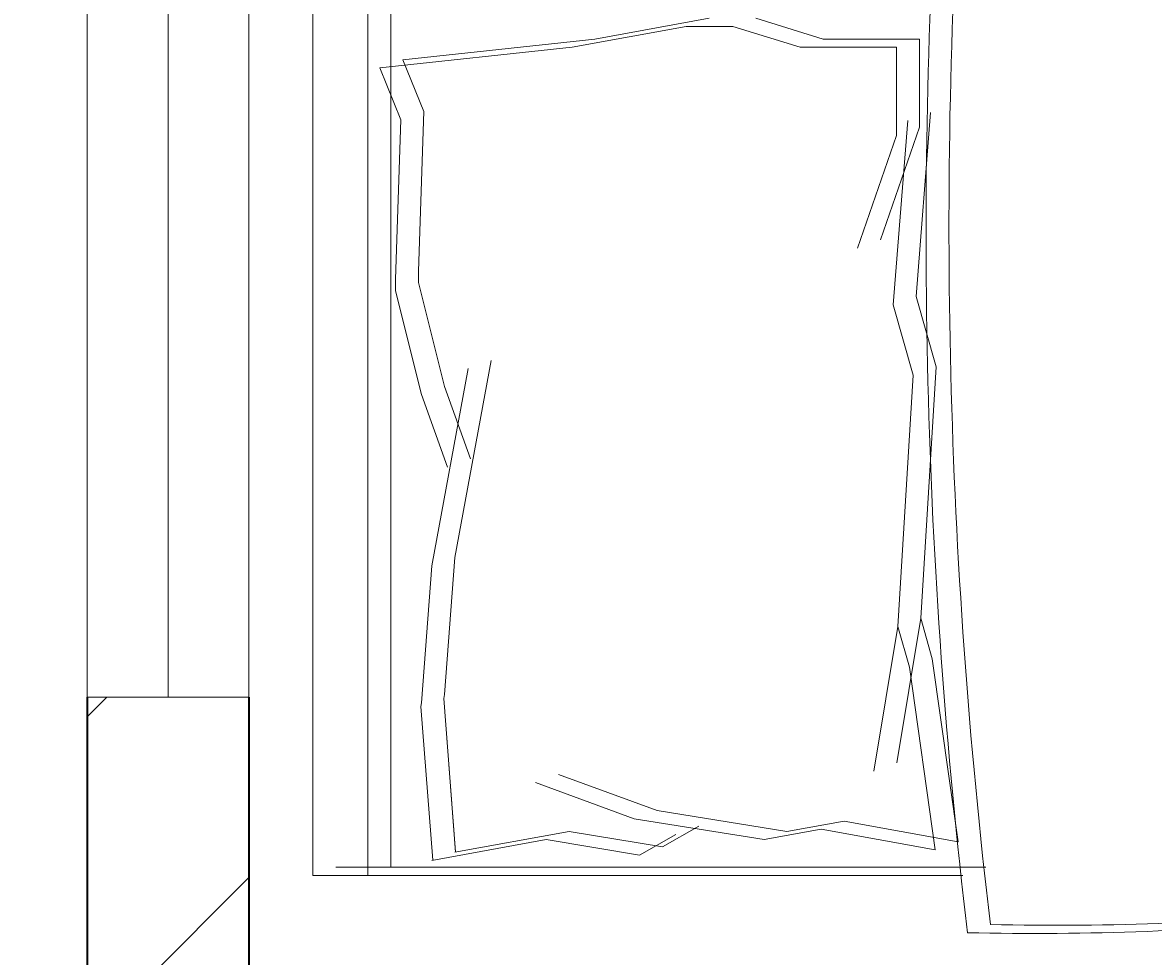
# Model space of a CAD drawing. Units: inches. Extents: x 1885 to 2748, y 783 to 2421.
# Tile 8 of 117: x 1969 to 2001, y 1138 to 1164. Entities that reach past the tile are written whole.
import ezdxf

# ---------------------------------------------------------------- set-up
doc = ezdxf.new("R2010")
doc.units = ezdxf.units.IN
for name, color, linetype, lineweight in [('A-ANNO-DIMS', 2, 'Continuous', 18), ('A-FURN', 8, 'Continuous', 13), ('A-GLAZ', 181, 'Continuous', 18), ('A-WALL', 7, 'Continuous', 35)]:
    doc.layers.add(name, color=color, linetype=linetype, lineweight=lineweight)
doc.layers.add('A-WALL-PATT', color=85, linetype='Continuous', lineweight=13, true_color=0x58ba48)
doc.styles.get("Standard").update_dxf_attribs({"font": 'arial.ttf'})
doc.dimstyles.get("Standard").update_dxf_attribs({"dimtxt": 0.18, "dimasz": 0.18, "dimexe": 0.18, "dimexo": 0.0625, "dimgap": 0.09, "dimtad": 0, "dimtih": 1, "dimtoh": 1, "dimdec": 4, "dimzin": 0, "dimdsep": 46, "dimtxsty": 'Standard', "dimcen": 0.09, "dimadec": 0, "dimazin": 0, "dimtfac": 1, "dimtdec": 4, "dimtofl": 0, "dimtmove": 0, "dimatfit": 3, "dimfxl": 1, "dimtolj": 1, "dimtzin": 0, "dimarcsym": 0})

# ---------------------------------------------------------------- blocks, each defined once
blk = doc.blocks.new('BED-DOUBLE')
for p, q in [((0.004, 3.474), (0.004, 51.493)), ((2.177, 3.702), (2.177, 51.493)), ((2.177, 3.702), (2.177, 51.492)), ((1.537, 3.474), (1.537, 51.264)), ((1.537, 3.474), (1.537, 51.264)), ((7.224, 26.56), (10.404, 27.138)), ((7.224, 26.559), (10.405, 27.137)), ((7.863, 26.788), (11.044, 27.366)), ((7.863, 26.788), (11.044, 27.366)), ((10.404, 27.138), (11.706, 27.138)), ((10.405, 27.137), (11.706, 27.137)), ((11.706, 27.138), (13.585, 26.56)), ((11.706, 27.137), (13.585, 26.559)), ((12.345, 27.366), (14.225, 26.788)), ((12.345, 27.366), (14.225, 26.788)), ((2.513, 26.21), (7.863, 26.788)), ((2.513, 26.209), (7.863, 26.788)), ((14.225, 26.788), (16.906, 26.788)), ((14.225, 26.788), (16.906, 26.788)), ((16.906, 26.788), (16.906, 24.33)), ((16.906, 26.788), (16.906, 24.33)), ((1.874, 25.981), (7.224, 26.56)), ((1.874, 25.981), (7.224, 26.559)), ((13.585, 26.56), (16.267, 26.56)), ((13.585, 26.559), (16.267, 26.559)), ((16.267, 26.56), (16.267, 24.102)), ((16.267, 26.559), (16.267, 24.102)), ((3.091, 24.764), (2.513, 26.21)), ((3.091, 24.764), (2.513, 26.209)), ((2.452, 24.536), (1.874, 25.981)), ((2.452, 24.535), (1.874, 25.981)), ((2.947, 20.319), (3.091, 24.764)), ((2.947, 20.318), (3.091, 24.764)), ((16.812, 19.611), (17.216, 24.743)), ((16.812, 19.611), (17.216, 24.743)), ((2.308, 20.09), (2.452, 24.536)), ((2.308, 20.09), (2.452, 24.535)), ((16.906, 24.33), (15.815, 21.186)), ((16.906, 24.33), (15.815, 21.186)), ((16.173, 19.383), (16.576, 24.515)), ((16.173, 19.382), (16.576, 24.514)), ((16.267, 24.102), (15.176, 20.957)), ((16.267, 24.102), (15.176, 20.957)), ((2.947, 19.997), (2.947, 20.319)), ((2.947, 19.997), (2.947, 20.318)), ((2.308, 19.769), (2.308, 20.09)), ((2.308, 19.768), (2.308, 20.09)), ((3.67, 17.106), (2.947, 19.997)), ((3.67, 17.105), (2.947, 19.997)), ((3.031, 16.877), (2.308, 19.769)), ((3.031, 16.877), (2.308, 19.768)), ((17.369, 17.651), (16.812, 19.611)), ((17.369, 17.65), (16.812, 19.611)), ((16.73, 17.422), (16.173, 19.383)), ((16.73, 17.422), (16.173, 19.382)), ((3.959, 12.335), (4.971, 17.829)), ((3.959, 12.335), (4.971, 17.828)), ((16.938, 10.641), (17.369, 17.651)), ((16.938, 10.64), (17.369, 17.65)), ((3.32, 12.107), (4.332, 17.6)), ((3.32, 12.107), (4.332, 17.6)), ((16.299, 10.412), (16.73, 17.422)), ((16.299, 10.412), (16.73, 17.422)), ((4.393, 15.082), (3.67, 17.106)), ((4.393, 15.082), (3.67, 17.105)), ((3.753, 14.854), (3.031, 16.877)), ((3.753, 14.853), (3.031, 16.877)), ((3.67, 8.512), (3.959, 12.335)), ((3.67, 8.512), (3.959, 12.335)), ((3.031, 8.284), (3.32, 12.107)), ((3.031, 8.283), (3.32, 12.107)), ((15.632, 6.38), (16.299, 10.412)), ((15.632, 6.38), (16.299, 10.412)), ((16.271, 6.609), (16.938, 10.641)), ((16.272, 6.609), (16.938, 10.64)), ((16.299, 10.412), (16.622, 9.279)), ((16.299, 10.412), (16.622, 9.279)), ((16.938, 10.641), (17.261, 9.508)), ((16.938, 10.64), (17.261, 9.507)), ((17.261, 9.508), (17.984, 4.411)), ((17.261, 9.507), (17.984, 4.411)), ((16.622, 9.279), (17.345, 4.183)), ((16.622, 9.279), (17.345, 4.182)), ((3.652, 8.407), (3.67, 8.512)), ((3.652, 8.406), (3.67, 8.512)), ((3.012, 8.178), (3.031, 8.284)), ((3.012, 8.178), (3.031, 8.283)), ((3.981, 4.126), (3.652, 8.407)), ((3.981, 4.125), (3.652, 8.406)), ((3.342, 3.897), (3.012, 8.178)), ((3.342, 3.897), (3.012, 8.178)), ((8.959, 5.05), (6.211, 6.062)), ((8.959, 5.05), (6.211, 6.061)), ((9.598, 5.278), (6.851, 6.29)), ((9.598, 5.278), (6.851, 6.29)), ((12.573, 4.472), (8.959, 5.05)), ((12.573, 4.471), (8.959, 5.05)), ((13.213, 4.7), (9.598, 5.278)), ((13.213, 4.7), (9.598, 5.278)), ((9.743, 4.266), (10.755, 4.845)), ((9.743, 4.266), (10.755, 4.844)), ((14.164, 4.761), (12.573, 4.472)), ((14.164, 4.76), (12.573, 4.471)), ((14.803, 4.989), (13.213, 4.7)), ((14.803, 4.989), (13.213, 4.7)), ((17.345, 4.183), (14.164, 4.761)), ((17.345, 4.182), (14.164, 4.76)), ((17.984, 4.411), (14.803, 4.989)), ((17.984, 4.411), (14.803, 4.989)), ((3.32, 3.893), (6.501, 4.472)), ((3.32, 3.893), (6.501, 4.471)), ((3.959, 4.122), (7.14, 4.7)), ((3.959, 4.121), (7.14, 4.7)), ((6.501, 4.472), (9.103, 4.038)), ((6.501, 4.471), (9.103, 4.038)), ((7.14, 4.7), (9.743, 4.266)), ((7.14, 4.7), (9.743, 4.266)), ((9.103, 4.038), (10.115, 4.616)), ((9.103, 4.038), (10.115, 4.616)), ((18.114, 3.474), (0.004, 3.474)), ((18.114, 3.474), (0.004, 3.474)), ((18.753, 3.702), (0.643, 3.702)), ((18.753, 3.702), (0.643, 3.702))]:
    blk.add_line(p, q)
for centre, radius, start, end in [((182.695, 21.586), 164.969, 176.08655, 186.78213), ((182.695, 21.586), 164.969, 176.08655, 186.78213), ((182.056, 21.358), 164.969, 176.08655, 186.78213), ((182.056, 21.357), 164.969, 176.08655, 186.78213), ((20.1, 85.16), 83.306, 268.72178, 275.60397), ((20.1, 85.16), 83.306, 268.72178, 275.60397), ((20.739, 85.389), 83.306, 268.72178, 275.60397), ((20.739, 85.389), 83.306, 268.72178, 275.60397)]:
    blk.add_arc(centre, radius, start, end)
blk = doc.blocks.new('WIN-60')
for p, q in [((0.004, 59.998), (0.004, -0.002)), ((2.254, 59.998), (2.254, -0.002)), ((4.504, -0.002), (4.504, 59.998)), ((2.254, -0.002), (0.004, -0.002)), ((0.004, -0.002), (4.504, -0.002))]:
    blk.add_line(p, q)
blk = doc.blocks.new('*D45')
at = {"layer": 'A-ANNO-DIMS', "color": 0, "lineweight": -2, "transparency": 16777216}
for p, q in [((1980.711, 1524.006), (1902.844, 1524.006)), ((1903.024, 1523.826), (1903.024, 1290.937)), ((1903.024, 1057.686), (1903.024, 1290.574)), ((1971.211, 1057.506), (1902.844, 1057.506))]:
    blk.add_line(p, q, dxfattribs=at)
at = {"layer": 'A-ANNO-DIMS', "color": 0, "transparency": 16777216}
for points in [[(1902.994, 1523.826), (1903.054, 1523.826), (1903.024, 1524.006)], [(1902.994, 1057.686), (1903.054, 1057.686), (1903.024, 1057.506)]]:
    blk.add_solid(points, dxfattribs=at)
at = {"layer": 'Defpoints', "color": 0, "transparency": 16777216}
for p in [(1903.024, 1524.006), (1980.774, 1524.006), (1971.274, 1057.506)]:
    blk.add_point(p, dxfattribs=at)
at = {"layer": 'A-ANNO-DIMS', "color": 0, "transparency": 16777216, "insert": (1903.024, 1290.756), "char_height": 0.18, "attachment_point": 5}
blk.add_mtext('\\A1;466.5', dxfattribs=at)

msp = doc.modelspace()

# ---------------------------------------------------------------- hatches: boundary and pattern name
at = {"layer": 'A-WALL-PATT'}
h = msp.add_hatch(dxfattribs=at)
h.set_pattern_fill('ANSI32', color=256)
h.paths.add_polyline_path([(2007.772, 2318.006), (1980.774, 2318.006), (1980.774, 2281.215), (1985.274, 2281.215), (1985.274, 2313.506), (2007.772, 2313.506), (2007.772, 2315.756)])
h.paths.add_polyline_path([(2094.324, 2318.006), (2067.772, 2318.006), (2067.772, 2313.506), (2094.324, 2313.506), (2094.324, 2315.756)])
h.paths.add_polyline_path([(2131.367, 2315.756), (2131.367, 2318.006), (2131.189, 2318.006), (2112.609, 2318.006), (2112.609, 2313.506), (2117.274, 2313.506), (2117.274, 2255.201), (2121.774, 2255.201), (2121.774, 2313.506), (2131.367, 2313.506)])
h.paths.add_polyline_path([(2190.512, 2318.006), (2155.367, 2318.006), (2155.367, 2313.506), (2169.774, 2313.506), (2169.774, 2229.506), (2121.774, 2229.506), (2121.774, 2233.451), (2119.524, 2233.451), (2117.274, 2233.451), (2117.274, 2201.101), (2121.774, 2201.101), (2121.774, 2225.006), (2169.774, 2225.006), (2169.774, 2165.006), (2306.274, 2165.006), (2306.274, 2066.006), (2310.774, 2066.006), (2344.274, 2066.006), (2486.274, 2066.006), (2486.274, 1886.006), (2483.02, 1886.006), (2483.02, 1881.506), (2486.274, 1881.506), (2486.274, 1880.678), (2490.774, 1880.678), (2490.774, 2070.506), (2344.274, 2070.506), (2310.774, 2070.506), (2310.774, 2165.006), (2310.774, 2173.636), (2308.524, 2173.636), (2306.274, 2173.636), (2306.274, 2169.506), (2174.274, 2169.506), (2174.274, 2313.506), (2190.512, 2313.506), (2190.512, 2315.756)])
h.paths.add_polyline_path([(1985.274, 2221.215), (1980.774, 2221.215), (1980.774, 2165.006), (1992.774, 2165.006), (1992.774, 2141.927), (1997.274, 2141.927), (1997.274, 2165.006), (2117.274, 2165.006), (2117.274, 2163.126), (2121.774, 2163.126), (2121.774, 2172.734), (2119.524, 2172.734), (2117.274, 2172.734), (2117.274, 2169.506), (1985.274, 2169.506)])
h.paths.add_polyline_path([(1997.274, 2105.927), (1992.774, 2105.927), (1992.774, 2070.506), (2016.774, 2070.506), (2016.774, 2059.123), (2019.024, 2059.123), (2021.274, 2059.123), (2021.274, 2070.506), (2117.274, 2070.506), (2117.274, 2022.506), (2114.423, 2022.506), (2114.423, 2018.006), (2123.627, 2018.006), (2123.627, 2020.256), (2123.627, 2022.506), (2121.774, 2022.506), (2121.774, 2142.587), (2119.524, 2142.587), (2117.274, 2142.587), (2117.274, 2075.006), (1997.274, 2075.006)])
h.paths.add_polyline_path([(2092.029, 2020.256), (2092.029, 2022.506), (2021.274, 2022.506), (2021.274, 2035.123), (2016.774, 2035.123), (2016.774, 2018.006), (2016.774, 1978.784), (2021.274, 1978.784), (2021.274, 2018.006), (2092.029, 2018.006)])
h.paths.add_polyline_path([(2260.938, 2022.506), (2153.105, 2022.506), (2153.105, 2020.256), (2153.105, 2018.006), (2155.274, 2018.006), (2155.274, 1886.006), (2107.629, 1886.006), (2107.629, 1881.506), (2182.911, 1881.506), (2182.911, 1883.756), (2182.911, 1886.006), (2159.774, 1886.006), (2159.774, 2018.006), (2260.938, 2018.006), (2260.938, 2020.256)])
h.paths.add_polyline_path([(2047.629, 1883.756), (2047.629, 1886.006), (2021.274, 1886.006), (2021.274, 1918.784), (2019.024, 1918.784), (2016.774, 1918.784), (2016.774, 1881.506), (2047.629, 1881.506)])
h.paths.add_polyline_path([(2306.361, 1883.756), (2306.361, 1886.006), (2296.274, 1886.006), (2296.274, 1982.006), (2316.535, 1982.006), (2316.535, 1984.256), (2316.535, 1986.506), (2296.274, 1986.506), (2296.274, 2022.506), (2289.276, 2022.506), (2289.276, 2018.006), (2291.774, 2018.006), (2291.774, 1886.006), (2242.911, 1886.006), (2242.911, 1881.506), (2306.361, 1881.506)], flags=17)
h.paths.add_polyline_path([(1985.274, 1843.006), (2021.6, 1843.006), (2021.534, 1845.441), (2021.477, 1847.506), (1980.774, 1847.506), (1980.774, 1809.446), (1985.274, 1809.446)])
h.paths.add_polyline_path([(2131.482, 1845.256), (2131.482, 1847.506), (2081.534, 1847.506), (2081.534, 1843.006), (2117.274, 1843.006), (2117.274, 1784.147), (2119.524, 1784.147), (2121.774, 1784.147), (2121.774, 1843.006), (2131.482, 1843.006)])
h.paths.add_polyline_path([(2203.886, 1847.506), (2155.482, 1847.506), (2155.482, 1843.006), (2169.774, 1843.006), (2169.774, 1759.006), (2121.774, 1759.006), (2121.774, 1761.457), (2117.274, 1761.457), (2117.274, 1730.429), (2121.774, 1730.429), (2121.774, 1754.506), (2177.421, 1754.506), (2177.421, 1756.756), (2177.421, 1759.006), (2174.274, 1759.006), (2174.274, 1843.006), (2203.886, 1843.006)])
h.paths.add_polyline_path([(2335.554, 1845.256), (2335.554, 1847.506), (2239.886, 1847.506), (2239.886, 1843.006), (2306.274, 1843.006), (2306.274, 1759.006), (2199.486, 1759.006), (2199.486, 1754.506), (2310.774, 1754.506), (2310.774, 1843.006), (2335.554, 1843.006)])
h.paths.add_polyline_path([(2348.774, 2022.506), (2344.274, 2022.506), (2344.274, 1986.506), (2341.681, 1986.506), (2341.681, 1982.006), (2344.274, 1982.006), (2344.274, 1886.006), (2330.361, 1886.006), (2330.361, 1881.506), (2361.627, 1881.506), (2361.627, 1883.756), (2361.627, 1886.006), (2348.774, 1886.006)], flags=17)
h.paths.add_polyline_path([(2283.251, 2315.756), (2283.251, 2318.006), (2238.512, 2318.006), (2238.512, 2313.506), (2283.251, 2313.506)], flags=17)
h.paths.add_polyline_path([(2363.274, 2348.006), (2388.677, 2348.006), (2388.677, 2350.256), (2388.677, 2352.506), (2358.774, 2352.506), (2358.774, 2348.006), (2358.774, 2318.006), (2344.481, 2318.006), (2344.481, 2313.506), (2358.774, 2313.506), (2358.774, 2229.506), (2310.774, 2229.506), (2310.774, 2231.952), (2306.274, 2231.952), (2306.274, 2205.611), (2310.774, 2205.611), (2310.774, 2225.006), (2358.774, 2225.006), (2358.774, 2211.506), (2452.329, 2211.506), (2452.329, 2213.756), (2452.329, 2216.006), (2363.274, 2216.006), (2363.274, 2318.006)])
h.paths.add_polyline_path([(2310.774, 2313.506), (2320.481, 2313.506), (2320.481, 2315.756), (2320.481, 2318.006), (2302.728, 2318.006), (2302.728, 2313.506), (2306.274, 2313.506), (2306.274, 2251.076), (2310.774, 2251.076)], flags=17)
h.paths.add_polyline_path([(2490.774, 2352.506), (2486.274, 2352.506), (2448.677, 2352.506), (2448.677, 2348.006), (2486.274, 2348.006), (2486.274, 2318.006), (2486.274, 2216.006), (2481.78, 2216.006), (2481.78, 2211.506), (2486.274, 2211.506), (2486.274, 2165.006), (2493.289, 2165.006), (2493.289, 2167.256), (2493.289, 2169.506), (2490.774, 2169.506), (2490.774, 2313.506), (2494.429, 2313.506), (2494.429, 2318.006), (2490.774, 2318.006)])
h.paths.add_polyline_path([(2534.653, 2318.006), (2515.691, 2318.006), (2515.691, 2313.506), (2534.653, 2313.506), (2534.653, 2315.756)])
h.paths.add_polyline_path([(2618.274, 2318.006), (2594.653, 2318.006), (2594.653, 2313.506), (2613.774, 2313.506), (2613.774, 2281.706), (2618.274, 2281.706)])
h.paths.add_polyline_path([(2618.274, 2221.706), (2613.774, 2221.706), (2613.774, 2169.506), (2554.019, 2169.506), (2554.019, 2165.006), (2613.774, 2165.006), (2613.774, 2152.878), (2618.274, 2152.878)])
h.paths.add_polyline_path([(2618.274, 2128.878), (2616.024, 2128.878), (2613.774, 2128.878), (2613.774, 2117.006), (2529.774, 2117.006), (2529.774, 2165.006), (2532.848, 2165.006), (2532.848, 2169.506), (2522.867, 2169.506), (2522.867, 2165.006), (2525.274, 2165.006), (2525.274, 2117.006), (2525.274, 2112.506), (2525.274, 2108.576), (2529.774, 2108.576), (2529.774, 2112.506), (2613.774, 2112.506), (2613.774, 2080.19), (2618.274, 2080.19)])
h.paths.add_polyline_path([(2618.274, 2044.19), (2616.024, 2044.19), (2613.774, 2044.19), (2613.774, 2015.506), (2529.774, 2015.506), (2529.774, 2088.582), (2527.524, 2088.582), (2525.274, 2088.582), (2525.274, 2011.006), (2613.774, 2011.006), (2613.774, 1956.755), (2618.274, 1956.755)])
h.paths.add_polyline_path([(2618.274, 1881.506), (2618.274, 1896.755), (2613.774, 1896.755), (2613.774, 1881.506), (2613.774, 1847.506), (2592.715, 1847.506), (2592.715, 1843.006), (2613.774, 1843.006), (2613.774, 1765.006), (2613.774, 1760.506), (2609.621, 1760.506), (2609.621, 1756.006), (2613.774, 1756.006), (2613.774, 1660.006), (2608.544, 1660.006), (2608.544, 1655.506), (2613.774, 1655.506), (2613.774, 1508.158), (2618.274, 1508.158)])
h.paths.add_polyline_path([(2565.774, 1843.006), (2568.997, 1843.006), (2568.997, 1847.506), (2490.774, 1847.506), (2490.774, 1849.7), (2488.524, 1849.7), (2486.274, 1849.7), (2486.274, 1847.506), (2477.274, 1847.506), (2477.274, 1838.506), (2477.274, 1821.493), (2486.274, 1821.493), (2486.274, 1838.506), (2561.274, 1838.506), (2561.274, 1765.006), (2486.274, 1765.006), (2486.274, 1786.157), (2477.274, 1786.157), (2477.274, 1765.006), (2477.274, 1756.006), (2486.274, 1756.006), (2565.774, 1756.006), (2585.621, 1756.006), (2585.621, 1758.256), (2585.621, 1760.506), (2565.774, 1760.506), (2565.774, 1765.006)])
h.paths.add_polyline_path([(2486.274, 1651.006), (2561.274, 1651.006), (2561.274, 1567.006), (2486.274, 1567.006), (2486.274, 1591.321), (2477.274, 1591.321), (2477.274, 1567.006), (2477.274, 1558.006), (2477.274, 1555.439), (2481.774, 1555.439), (2481.774, 1558.006), (2568.653, 1558.006), (2568.653, 1560.256), (2568.653, 1562.506), (2565.774, 1562.506), (2565.774, 1655.506), (2584.544, 1655.506), (2584.544, 1657.756), (2584.544, 1660.006), (2565.774, 1660.006), (2486.274, 1660.006), (2477.274, 1660.006), (2477.274, 1651.006), (2477.274, 1632.989), (2486.274, 1632.989)])
h.paths.add_polyline_path([(2449.967, 1883.756), (2449.967, 1886.006), (2421.627, 1886.006), (2421.627, 1881.506), (2449.967, 1881.506)], flags=17)
h.paths.add_polyline_path([(2447.274, 1847.506), (2395.554, 1847.506), (2395.554, 1843.006), (2442.774, 1843.006), (2442.774, 1809.27), (2447.274, 1809.27)])
h.paths.add_polyline_path([(1985.274, 1749.446), (1980.774, 1749.446), (1980.774, 1694.504), (1985.274, 1694.504), (1985.274, 1694.506), (1986.897, 1694.506), (1986.897, 1697.78), (1986.897, 1699.006), (1985.274, 1699.006)])
h.paths.add_polyline_path([(2152.774, 1699.006), (2121.774, 1699.006), (2121.774, 1703.668), (2119.524, 1703.668), (2117.274, 1703.668), (2117.274, 1699.006), (2009.219, 1699.006), (2009.219, 1694.506), (2148.274, 1694.506), (2148.274, 1692.631), (2152.774, 1692.631)])
h.paths.add_polyline_path([(2016.274, 1694.506), (2011.774, 1694.506), (2011.774, 1558.006), (2040.806, 1558.006), (2040.806, 1560.256), (2040.806, 1562.506), (2016.274, 1562.506)])
h.paths.add_polyline_path([(2152.774, 1663.017), (2150.524, 1663.017), (2148.274, 1663.017), (2148.274, 1562.506), (2100.806, 1562.506), (2100.806, 1558.006), (2165.119, 1558.006), (2165.119, 1560.256), (2165.119, 1562.506), (2152.774, 1562.506), (2152.774, 1610.506), (2224.774, 1610.506), (2224.774, 1607.99), (2229.274, 1607.99), (2229.274, 1615.006), (2152.774, 1615.006)])
h.paths.add_polyline_path([(2238.613, 1560.256), (2238.613, 1562.506), (2229.274, 1562.506), (2229.274, 1588.756), (2227.024, 1588.763), (2224.774, 1588.771), (2224.774, 1562.506), (2189.119, 1562.506), (2189.119, 1558.006), (2238.613, 1558.006)])
h.paths.add_polyline_path([(2336.024, 1560.256), (2336.024, 1562.506), (2310.774, 1562.506), (2310.774, 1656.347), (2308.524, 1656.347), (2306.274, 1656.347), (2306.274, 1562.506), (2286.613, 1562.506), (2286.613, 1558.006), (2336.024, 1558.006)])
h.paths.add_polyline_path([(2447.274, 1690.968), (2445.024, 1690.968), (2442.774, 1690.968), (2442.774, 1687.006), (2306.274, 1687.006), (2306.274, 1680.75), (2310.774, 1680.75), (2310.774, 1682.506), (2442.774, 1682.506), (2442.774, 1562.506), (2396.024, 1562.506), (2396.024, 1558.006), (2447.274, 1558.006)])
h.paths.add_polyline_path([(2447.274, 1749.27), (2445.024, 1749.27), (2442.774, 1749.27), (2442.774, 1717.232), (2447.274, 1717.232)])
h.paths.add_polyline_path([(2044.674, 1521.756), (2044.674, 1524.006), (2007.274, 1524.006), (2007.274, 1503.49), (2009.524, 1503.49), (2011.774, 1503.49), (2011.774, 1519.506), (2044.674, 1519.506)])
h.paths.add_polyline_path([(2177.969, 1521.756), (2177.969, 1524.006), (2104.674, 1524.006), (2104.674, 1519.506), (2145.774, 1519.506), (2145.774, 1387.506), (2143.37, 1387.506), (2143.37, 1383.006), (2251.585, 1383.006), (2251.585, 1385.256), (2251.585, 1387.506), (2150.274, 1387.506), (2150.274, 1519.506), (2177.969, 1519.506)])
h.paths.add_polyline_path([(2298.704, 1524.006), (2237.969, 1524.006), (2237.969, 1519.506), (2282.274, 1519.506), (2282.274, 1387.506), (2279.683, 1387.506), (2279.683, 1383.006), (2286.774, 1383.006), (2286.774, 1419.006), (2312.451, 1419.006), (2312.451, 1421.256), (2312.451, 1423.506), (2286.774, 1423.506), (2286.774, 1519.506), (2298.704, 1519.506), (2298.704, 1521.722)], flags=17)
h.paths.add_polyline_path([(2361.897, 1521.756), (2361.897, 1524.006), (2322.704, 1524.006), (2322.704, 1519.506), (2334.774, 1519.506), (2334.774, 1423.506), (2331.93, 1423.506), (2331.93, 1419.006), (2334.774, 1419.006), (2334.774, 1387.506), (2334.774, 1383.228), (2339.274, 1383.228), (2339.274, 1387.506), (2339.274, 1519.506), (2361.897, 1519.506)], flags=17)
h.paths.add_polyline_path([(2447.274, 1521.756), (2447.274, 1524.006), (2421.897, 1524.006), (2421.897, 1519.506), (2447.274, 1519.506)], flags=17)
h.paths.add_polyline_path([(2481.774, 1529.6), (2479.524, 1529.6), (2477.274, 1529.6), (2477.274, 1524.006), (2474.489, 1524.006), (2474.489, 1519.506), (2477.274, 1519.506), (2477.274, 1334.506), (2296.774, 1334.506), (2296.774, 1240.506), (2160.274, 1240.506), (2160.274, 1180.506), (2112.274, 1180.506), (2112.274, 1207.692), (2110.024, 1207.692), (2107.774, 1207.692), (2107.774, 1171.609), (2112.274, 1171.609), (2112.274, 1176.006), (2160.274, 1176.006), (2160.274, 1092.006), (2144.221, 1092.006), (2144.221, 1087.506), (2189.497, 1087.506), (2189.497, 1089.756), (2189.497, 1092.006), (2164.774, 1092.006), (2164.774, 1236.006), (2296.774, 1236.006), (2296.774, 1231.912), (2301.274, 1231.912), (2301.274, 1330.006), (2481.774, 1330.006), (2481.774, 1387.506)])
h.paths.add_polyline_path([(2618.274, 1448.158), (2613.774, 1448.158), (2613.774, 1382.506), (2529.774, 1382.506), (2525.274, 1382.506), (2525.274, 1307.062), (2529.774, 1307.062), (2529.774, 1378.006), (2613.774, 1378.006), (2613.774, 1354.988), (2618.274, 1354.988)])
h.paths.add_polyline_path([(2618.274, 1318.988), (2613.774, 1318.988), (2613.774, 1281.006), (2529.774, 1281.006), (2529.774, 1283.786), (2527.524, 1283.786), (2525.274, 1283.786), (2525.274, 1228.506), (2516.794, 1228.506), (2516.794, 1224.006), (2533.484, 1224.006), (2533.484, 1226.256), (2533.484, 1228.506), (2529.774, 1228.506), (2529.774, 1276.506), (2613.774, 1276.506), (2613.774, 1266.02), (2618.274, 1266.02)])
h.paths.add_polyline_path([(2618.274, 1134.964), (2613.774, 1134.964), (2613.774, 1092.006), (2594.545, 1092.006), (2594.545, 1087.506), (2618.274, 1087.506)])
h.paths.add_polyline_path([(2534.545, 1092.006), (2509.765, 1092.006), (2509.765, 1087.506), (2534.545, 1087.506), (2534.545, 1089.756)])
h.paths.add_polyline_path([(2481.274, 1224.006), (2484.117, 1224.006), (2484.117, 1226.256), (2484.117, 1228.506), (2476.774, 1228.506), (2476.774, 1198.506), (2471.61, 1198.506), (2471.61, 1194.006), (2476.774, 1194.006), (2476.774, 1062.006), (2436.894, 1062.006), (2436.894, 1057.506), (2476.774, 1057.506), (2481.274, 1057.506), (2481.274, 1062.006), (2481.274, 1087.506), (2485.354, 1087.506), (2485.354, 1089.756), (2485.354, 1092.006), (2481.274, 1092.006), (2481.274, 1117.506)])
h.paths.add_polyline_path([(2439.898, 1198.506), (2349.274, 1198.506), (2349.274, 1194.006), (2349.274, 1180.506), (2301.274, 1180.506), (2301.274, 1201.896), (2299.024, 1201.896), (2296.774, 1201.896), (2296.774, 1172.335), (2299.024, 1172.335), (2301.274, 1172.335), (2301.274, 1176.006), (2349.274, 1176.006), (2349.274, 1092.006), (2334.452, 1092.006), (2334.452, 1087.506), (2349.274, 1087.506), (2349.274, 1057.506), (2353.774, 1057.506), (2376.894, 1057.506), (2376.894, 1059.756), (2376.894, 1062.006), (2353.774, 1062.006), (2353.774, 1087.506), (2353.774, 1180.506), (2353.774, 1194.006), (2439.898, 1194.006), (2439.898, 1196.256)])
h.paths.add_polyline_path([(2270.596, 1089.756), (2270.596, 1092.006), (2249.497, 1092.006), (2249.497, 1087.506), (2270.596, 1087.506)], flags=17)
h.paths.add_polyline_path([(2310.452, 1092.006), (2301.274, 1092.006), (2301.274, 1153.292), (2296.774, 1153.292), (2296.774, 1092.006), (2293.786, 1092.006), (2293.786, 1087.506), (2310.452, 1087.506), (2310.452, 1089.756)], flags=17)
h.paths.add_polyline_path([(2112.274, 1150.328), (2110.024, 1150.328), (2107.774, 1150.328), (2107.774, 1092.006), (2104.465, 1092.006), (2104.465, 1087.506), (2120.221, 1087.506), (2120.221, 1089.756), (2120.221, 1092.006), (2112.274, 1092.006)])
h.paths.add_polyline_path([(2082.172, 1092.006), (2058.144, 1092.006), (2058.144, 1087.506), (2082.172, 1087.506), (2082.172, 1089.756)])
h.paths.add_polyline_path([(1975.774, 1145.638), (1971.274, 1145.638), (1971.274, 1087.506), (1980.774, 1087.506), (1998.144, 1087.506), (1998.144, 1089.756), (1998.144, 1092.006), (1985.274, 1092.006), (1975.774, 1092.006)])
h.paths.add_polyline_path([(2112.274, 1244.385), (2110.024, 1244.385), (2107.774, 1244.385), (2107.774, 1240.506), (1992.274, 1240.506), (1992.274, 1271.008), (1987.774, 1271.008), (1987.774, 1240.506), (1980.774, 1240.506), (1975.774, 1240.506), (1971.274, 1240.506), (1971.274, 1205.638), (1975.774, 1205.638), (1975.774, 1236.006), (2107.774, 1236.006), (2107.774, 1233.444), (2112.274, 1233.444), (2112.274, 1236.006)])
h.paths.add_polyline_path([(2112.274, 1383.006), (2114.783, 1383.006), (2114.783, 1385.256), (2114.783, 1387.506), (2102.476, 1387.506), (2102.476, 1383.006), (2107.774, 1383.006), (2107.774, 1335.006), (2011.774, 1335.006), (2011.774, 1349.939), (2007.274, 1349.939), (2007.274, 1335.006), (1987.774, 1335.006), (1987.774, 1330.506), (1987.774, 1307.008), (1992.274, 1307.008), (1992.274, 1330.506), (2007.274, 1330.506), (2107.774, 1330.506), (2107.774, 1264.711), (2112.274, 1264.711)])
h.paths.add_polyline_path([(2077.857, 1387.506), (2011.774, 1387.506), (2011.774, 1390.036), (2009.524, 1390.036), (2007.274, 1390.036), (2007.274, 1373.939), (2011.774, 1373.939), (2011.774, 1383.006), (2077.857, 1383.006)])
h.paths.add_polyline_path([(2011.774, 1443.49), (2007.274, 1443.49), (2007.274, 1410.248), (2011.774, 1410.248)])

# ---------------------------------------------------------------- linework, layer by layer
at = {"layer": 'A-WALL'}
for p, q in [((1971.274, 1145.638), (1971.274, 1087.506)), ((1975.774, 1145.638), (1975.774, 1092.006))]:
    msp.add_line(p, q, dxfattribs=at)

# ---------------------------------------------------------------- block references
at = {"layer": 'A-FURN'}
msp.add_blockref('BED-DOUBLE', (1977.555, 1137.199), dxfattribs=at)
at = {"layer": 'A-GLAZ'}
msp.add_blockref('WIN-60', (1971.27, 1145.64), dxfattribs=at)

# ---------------------------------------------------------------- dimensions: what is measured, and where the dimension line sits
at = {"layer": 'A-ANNO-DIMS'}
dim = msp.add_linear_dim(base=(1903.024, 1524.006), p1=(1971.274, 1057.506), p2=(1980.774, 1524.006), angle=90, dimstyle='Standard', override={"dimdec": 1, "dimlfac": 1, "dimrnd": 0, "dimzin": 0, "dimdsep": 46, "dimlunit": 2}, dxfattribs=at)
dim.commit()
dim.dimension.update_dxf_attribs({"geometry": '*D45', "text_midpoint": (1903.024, 1290.756)})

doc.saveas('drawing.dxf')
